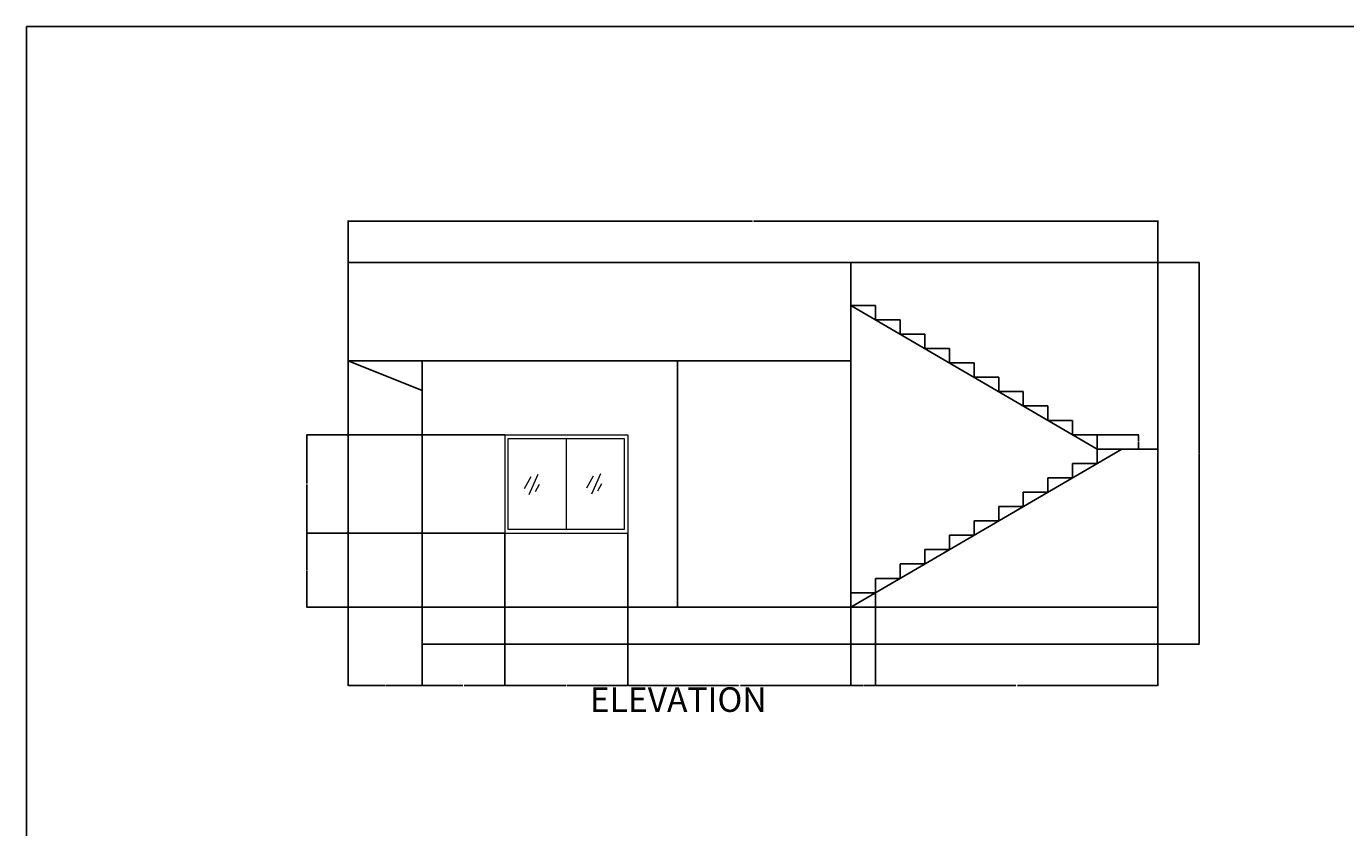
# Model space of a CAD drawing. Units: inches. Extents: x 1587 to 2880, y 1287 to 2423.
# Tile 5 of 8: x 1587 to 2229, y 2033 to 2423. Entities that reach past the tile are written whole.
import ezdxf

# ---------------------------------------------------------------- set-up
doc = ezdxf.new("R2010")
doc.units = ezdxf.units.IN
for name, color, linetype, lineweight in [('A-ANNO-DIMS', 2, 'Continuous', 18), ('A-ANNO-TEXT', 7, 'Continuous', 18), ('A-ANNO-TTLB', 7, 'Continuous', 25), ('A-ELEV', 7, 'Continuous', 25), ('A-FLOR-STRS', 7, 'Continuous', 25), ('A-GLAZ', 4, 'Continuous', 18)]:
    doc.layers.add(name, color=color, linetype=linetype, lineweight=lineweight)
doc.layers.add('A-WALL-PATT', color=251, linetype='Continuous', lineweight=13, true_color=0x636466)
doc.styles.get("Standard").update_dxf_attribs({"font": 'arial.ttf'})
doc.dimstyles.get("Standard").update_dxf_attribs({"dimtxt": 0.18, "dimasz": 0.18, "dimexe": 0.18, "dimexo": 0.0625, "dimgap": 0.09, "dimtad": 0, "dimtih": 1, "dimtoh": 1, "dimdec": 4, "dimzin": 0, "dimdsep": 46, "dimtxsty": 'Standard', "dimcen": 0.09, "dimadec": 0, "dimazin": 0, "dimtfac": 1, "dimtdec": 4, "dimtofl": 0, "dimtmove": 0, "dimatfit": 3, "dimfxl": 1, "dimtolj": 1, "dimtzin": 0, "dimarcsym": 0})

# ---------------------------------------------------------------- blocks, each defined once
blk = doc.blocks.new('GLASS-REFLECTION-ELEV')
for p, q in [((3.25, 8.8), (0, 2.81)), ((6.7, 9.88), (2.36, 0)), ((7.34, 5.04), (5.36, 1.47))]:
    blk.add_line(p, q)
blk = doc.blocks.new('*D82')
at = {"layer": 'A-ANNO-DIMS', "color": 0, "lineweight": -2, "transparency": 16777216}
for p, q in [((1743.34, 2308.21), (1743.34, 2328.48)), ((1743.52, 2328.3), (1940.2, 2328.3)), ((2137.66, 2328.3), (1940.99, 2328.3)), ((2137.84, 2308.21), (2137.84, 2328.48))]:
    blk.add_line(p, q, dxfattribs=at)
at = {"layer": 'A-ANNO-DIMS', "color": 0, "transparency": 16777216}
for points in [[(1743.52, 2328.33), (1743.52, 2328.27), (1743.34, 2328.3)], [(2137.66, 2328.33), (2137.66, 2328.27), (2137.84, 2328.3)]]:
    blk.add_solid(points, dxfattribs=at)
at = {"layer": 'Defpoints', "color": 0, "transparency": 16777216}
for p in [(2137.84, 2328.3), (1743.34, 2308.15), (2137.84, 2308.15)]:
    blk.add_point(p, dxfattribs=at)
at = {"layer": 'A-ANNO-DIMS', "color": 0, "transparency": 16777216, "insert": (1940.59, 2328.3), "char_height": 0.18, "attachment_point": 5}
blk.add_mtext('\\A1;394.5', dxfattribs=at)
blk = doc.blocks.new('*D83')
at = {"layer": 'A-ANNO-DIMS', "color": 0, "lineweight": -2, "transparency": 16777216}
for p, q in [((2137.9, 2308.15), (2158.17, 2308.15)), ((2157.99, 2307.97), (2157.99, 2215.33)), ((2157.99, 2122.33), (2157.99, 2214.97)), ((2137.9, 2122.15), (2158.17, 2122.15))]:
    blk.add_line(p, q, dxfattribs=at)
at = {"layer": 'A-ANNO-DIMS', "color": 0, "transparency": 16777216}
for points in [[(2157.96, 2307.97), (2158.02, 2307.97), (2157.99, 2308.15)], [(2157.96, 2122.33), (2158.02, 2122.33), (2157.99, 2122.15)]]:
    blk.add_solid(points, dxfattribs=at)
at = {"layer": 'Defpoints', "color": 0, "transparency": 16777216}
for p in [(2137.84, 2308.15), (2157.99, 2308.15), (2137.84, 2122.15)]:
    blk.add_point(p, dxfattribs=at)
at = {"layer": 'A-ANNO-DIMS', "color": 0, "transparency": 16777216, "insert": (2157.99, 2215.15), "char_height": 0.18, "attachment_point": 5}
blk.add_mtext('\\A1;186', dxfattribs=at)
blk = doc.blocks.new('*D84')
at = {"layer": 'A-ANNO-DIMS', "color": 0, "lineweight": -2, "transparency": 16777216}
for p, q in [((1743.34, 2260.09), (1743.34, 2101.82)), ((1779.34, 2122.09), (1779.34, 2101.82)), ((1743.52, 2102), (1761.12, 2102)), ((1779.16, 2102), (1761.56, 2102))]:
    blk.add_line(p, q, dxfattribs=at)
at = {"layer": 'A-ANNO-DIMS', "color": 0, "transparency": 16777216}
for points in [[(1743.52, 2102.03), (1743.52, 2101.97), (1743.34, 2102)], [(1779.16, 2102.03), (1779.16, 2101.97), (1779.34, 2102)]]:
    blk.add_solid(points, dxfattribs=at)
at = {"layer": 'Defpoints', "color": 0, "transparency": 16777216}
for p in [(1743.34, 2260.15), (1779.34, 2122.15), (1779.34, 2102)]:
    blk.add_point(p, dxfattribs=at)
at = {"layer": 'A-ANNO-DIMS', "color": 0, "transparency": 16777216, "insert": (1761.34, 2102), "char_height": 0.18, "attachment_point": 5}
blk.add_mtext('\\A1;36', dxfattribs=at)
blk = doc.blocks.new('*D85')
at = {"layer": 'A-ANNO-DIMS', "color": 0, "lineweight": -2, "transparency": 16777216}
for p, q in [((1819.66, 2176.09), (1819.66, 2101.82)), ((1779.34, 2140.09), (1779.34, 2101.82)), ((1779.52, 2102), (1799.11, 2102)), ((1819.48, 2102), (1799.9, 2102))]:
    blk.add_line(p, q, dxfattribs=at)
at = {"layer": 'A-ANNO-DIMS', "color": 0, "transparency": 16777216}
for points in [[(1779.52, 2102.03), (1779.52, 2101.97), (1779.34, 2102)], [(1819.48, 2102.03), (1819.48, 2101.97), (1819.66, 2102)]]:
    blk.add_solid(points, dxfattribs=at)
at = {"layer": 'Defpoints', "color": 0, "transparency": 16777216}
for p in [(1819.66, 2176.15), (1779.34, 2140.15), (1819.66, 2102)]:
    blk.add_point(p, dxfattribs=at)
at = {"layer": 'A-ANNO-DIMS', "color": 0, "transparency": 16777216, "insert": (1799.5, 2102), "char_height": 0.18, "attachment_point": 5}
blk.add_mtext('\\A1;40.32', dxfattribs=at)
blk = doc.blocks.new('*D86')
at = {"layer": 'A-ANNO-DIMS', "color": 0, "lineweight": -2, "transparency": 16777216}
for p, q in [((1819.66, 2176.09), (1819.66, 2101.82)), ((1879.66, 2176.09), (1879.66, 2101.82)), ((1819.84, 2102), (1849.44, 2102)), ((1879.48, 2102), (1849.88, 2102))]:
    blk.add_line(p, q, dxfattribs=at)
at = {"layer": 'A-ANNO-DIMS', "color": 0, "transparency": 16777216}
for points in [[(1819.84, 2102.03), (1819.84, 2101.97), (1819.66, 2102)], [(1879.48, 2102.03), (1879.48, 2101.97), (1879.66, 2102)]]:
    blk.add_solid(points, dxfattribs=at)
at = {"layer": 'Defpoints', "color": 0, "transparency": 16777216}
for p in [(1819.66, 2176.15), (1879.66, 2176.15), (1879.66, 2102)]:
    blk.add_point(p, dxfattribs=at)
at = {"layer": 'A-ANNO-DIMS', "color": 0, "transparency": 16777216, "insert": (1849.66, 2102), "char_height": 0.18, "attachment_point": 5}
blk.add_mtext('\\A1;60', dxfattribs=at)
blk = doc.blocks.new('*D87')
at = {"layer": 'A-ANNO-DIMS', "color": 0, "lineweight": -2, "transparency": 16777216}
for p, q in [((1879.66, 2176.09), (1879.66, 2101.82)), ((1988.29, 2140.09), (1988.29, 2101.82)), ((1879.84, 2102), (1933.52, 2102)), ((1988.11, 2102), (1934.43, 2102))]:
    blk.add_line(p, q, dxfattribs=at)
at = {"layer": 'A-ANNO-DIMS', "color": 0, "transparency": 16777216}
for points in [[(1879.84, 2102.03), (1879.84, 2101.97), (1879.66, 2102)], [(1988.11, 2102.03), (1988.11, 2101.97), (1988.29, 2102)]]:
    blk.add_solid(points, dxfattribs=at)
at = {"layer": 'Defpoints', "color": 0, "transparency": 16777216}
for p in [(1879.66, 2176.15), (1988.29, 2140.15), (1988.29, 2102)]:
    blk.add_point(p, dxfattribs=at)
at = {"layer": 'A-ANNO-DIMS', "color": 0, "transparency": 16777216, "insert": (1933.98, 2102), "char_height": 0.18, "attachment_point": 5}
blk.add_mtext('\\A1;108.63', dxfattribs=at)
blk = doc.blocks.new('*D88')
at = {"layer": 'A-ANNO-DIMS', "color": 0, "lineweight": -2, "transparency": 16777216}
for p, q in [((1819.6, 2224.15), (1723.01, 2224.15)), ((1723.19, 2223.97), (1723.19, 2200.33)), ((1723.19, 2176.33), (1723.19, 2199.97)), ((1819.6, 2176.15), (1723.01, 2176.15))]:
    blk.add_line(p, q, dxfattribs=at)
at = {"layer": 'A-ANNO-DIMS', "color": 0, "transparency": 16777216}
for points in [[(1723.16, 2223.97), (1723.22, 2223.97), (1723.19, 2224.15)], [(1723.16, 2176.33), (1723.22, 2176.33), (1723.19, 2176.15)]]:
    blk.add_solid(points, dxfattribs=at)
at = {"layer": 'Defpoints', "color": 0, "transparency": 16777216}
for p in [(1723.19, 2224.15), (1819.66, 2224.15), (1819.66, 2176.15)]:
    blk.add_point(p, dxfattribs=at)
at = {"layer": 'A-ANNO-DIMS', "color": 0, "transparency": 16777216, "insert": (1723.19, 2200.15), "char_height": 0.18, "attachment_point": 5}
blk.add_mtext('\\A1;48', dxfattribs=at)
blk = doc.blocks.new('*D89')
at = {"layer": 'A-ANNO-DIMS', "color": 0, "lineweight": -2, "transparency": 16777216}
for p, q in [((1819.6, 2176.15), (1723.01, 2176.15)), ((1723.19, 2175.97), (1723.19, 2158.33)), ((1723.19, 2140.33), (1723.19, 2157.97)), ((1779.28, 2140.15), (1723.01, 2140.15))]:
    blk.add_line(p, q, dxfattribs=at)
at = {"layer": 'A-ANNO-DIMS', "color": 0, "transparency": 16777216}
for points in [[(1723.16, 2175.97), (1723.22, 2175.97), (1723.19, 2176.15)], [(1723.16, 2140.33), (1723.22, 2140.33), (1723.19, 2140.15)]]:
    blk.add_solid(points, dxfattribs=at)
at = {"layer": 'Defpoints', "color": 0, "transparency": 16777216}
for p in [(1723.19, 2176.15), (1819.66, 2176.15), (1779.34, 2140.15)]:
    blk.add_point(p, dxfattribs=at)
at = {"layer": 'A-ANNO-DIMS', "color": 0, "transparency": 16777216, "insert": (1723.19, 2158.15), "char_height": 0.18, "attachment_point": 5}
blk.add_mtext('\\A1;36', dxfattribs=at)
blk = doc.blocks.new('*D90')
at = {"layer": 'A-ANNO-DIMS', "color": 0, "lineweight": -2, "transparency": 16777216}
for p, q in [((1988.29, 2147.09), (1988.29, 2101.82)), ((2000.29, 2147.09), (2000.29, 2101.82)), ((1988.47, 2102), (1994.08, 2102)), ((2000.11, 2102), (1994.5, 2102))]:
    blk.add_line(p, q, dxfattribs=at)
at = {"layer": 'A-ANNO-DIMS', "color": 0, "transparency": 16777216}
for points in [[(1988.47, 2102.03), (1988.47, 2101.97), (1988.29, 2102)], [(2000.11, 2102.03), (2000.11, 2101.97), (2000.29, 2102)]]:
    blk.add_solid(points, dxfattribs=at)
at = {"layer": 'Defpoints', "color": 0, "transparency": 16777216}
for p in [(1988.29, 2147.15), (2000.29, 2147.15), (2000.29, 2102)]:
    blk.add_point(p, dxfattribs=at)
at = {"layer": 'A-ANNO-DIMS', "color": 0, "transparency": 16777216, "insert": (1994.29, 2102), "char_height": 0.18, "attachment_point": 5}
blk.add_mtext('\\A1;12', dxfattribs=at)
blk = doc.blocks.new('*D91')
at = {"layer": 'A-ANNO-DIMS', "color": 0, "lineweight": -2, "transparency": 16777216}
for p, q in [((2000.29, 2147.09), (2000.29, 2101.82)), ((2137.84, 2140.09), (2137.84, 2101.82)), ((2000.47, 2102), (2068.61, 2102)), ((2137.66, 2102), (2069.52, 2102))]:
    blk.add_line(p, q, dxfattribs=at)
at = {"layer": 'A-ANNO-DIMS', "color": 0, "transparency": 16777216}
for points in [[(2000.47, 2102.03), (2000.47, 2101.97), (2000.29, 2102)], [(2137.66, 2102.03), (2137.66, 2101.97), (2137.84, 2102)]]:
    blk.add_solid(points, dxfattribs=at)
at = {"layer": 'Defpoints', "color": 0, "transparency": 16777216}
for p in [(2000.29, 2147.15), (2137.84, 2140.15), (2137.84, 2102)]:
    blk.add_point(p, dxfattribs=at)
at = {"layer": 'A-ANNO-DIMS', "color": 0, "transparency": 16777216, "insert": (2069.07, 2102), "char_height": 0.18, "attachment_point": 5}
blk.add_mtext('\\A1;137.55', dxfattribs=at)
blk = doc.blocks.new('*D92')
at = {"layer": 'A-ANNO-DIMS', "color": 0, "lineweight": -2, "transparency": 16777216}
for p, q in [((2108.356572, 2224.151475), (2128.624072, 2224.151475)), ((2128.444072, 2223.971475), (2128.444072, 2220.831475)), ((2128.444072, 2217.331475), (2128.444072, 2220.471475)), ((2108.356572, 2217.151475), (2128.624072, 2217.151475))]:
    blk.add_line(p, q, dxfattribs=at)
at = {"layer": 'A-ANNO-DIMS', "color": 0, "transparency": 16777216}
for points in [[(2128.414072, 2223.971475), (2128.474072, 2223.971475), (2128.444072, 2224.151475)], [(2128.414072, 2217.331475), (2128.474072, 2217.331475), (2128.444072, 2217.151475)]]:
    blk.add_solid(points, dxfattribs=at)
at = {"layer": 'Defpoints', "color": 0, "transparency": 16777216}
for p in [(2108.294072, 2224.151475), (2108.294072, 2217.151475), (2128.444072, 2217.151475)]:
    blk.add_point(p, dxfattribs=at)
at = {"layer": 'A-ANNO-DIMS', "color": 0, "transparency": 16777216, "insert": (2128.444072, 2220.651475), "char_height": 0.18, "attachment_point": 5}
blk.add_mtext('\\A1;7', dxfattribs=at)

msp = doc.modelspace()

# ---------------------------------------------------------------- hatches: boundary and pattern name
at = {"layer": 'A-WALL-PATT'}
h = msp.add_hatch(color=256, dxfattribs=at)
h.dxf.hatch_style = 1
h.paths.add_polyline_path([(2190.3423, 1988.3868), (2181.3423, 1988.3868), (2137.8423, 1988.3868), (1779.3423, 1988.3868), (1779.3423, 1939.6287), (1788.3423, 1939.6287), (1788.3423, 1979.3868), (1956.3423, 1979.3868), (1956.3423, 1841.3868), (1948.4175, 1841.3868), (1948.4175, 1836.8868), (1968.256, 1836.8868), (1968.256, 1839.1368), (1968.256, 1841.3868), (1960.8423, 1841.3868), (1960.8423, 1979.3868), (2128.8423, 1979.3868), (2128.8423, 1971.4394), (2133.3423, 1971.4394), (2133.3423, 1979.3868), (2181.3423, 1979.3868), (2181.3423, 1895.3868), (2174.9842, 1895.3868), (2174.9842, 1886.3868), (2190.3423, 1886.3868), (2190.3423, 1895.3868)])
h.paths.add_polyline_path([(1788.3423, 1879.6287), (1779.3423, 1879.6287), (1779.3423, 1827.4437), (1788.3423, 1827.4437), (1788.3423, 1836.8868), (1839.8915, 1836.8868), (1839.8915, 1839.1368), (1839.8915, 1841.3868), (1788.3423, 1841.3868)])
h.paths.add_polyline_path([(1876.8423, 1836.8868), (1908.901, 1836.8868), (1908.901, 1839.1368), (1908.901, 1841.3868), (1866.9993, 1841.3868), (1866.9993, 1836.8868), (1872.3423, 1836.8868), (1872.3423, 1776.8868), (1788.3423, 1776.8868), (1788.3423, 1803.4437), (1779.3423, 1803.4437), (1779.3423, 1757.1447), (1788.3423, 1757.1447), (1788.3423, 1772.3868), (1872.3423, 1772.3868), (1872.3423, 1712.3868), (1867.9542, 1712.3868), (1867.9542, 1707.8868), (1876.8423, 1707.8868), (1876.8423, 1772.3868)])
h.paths.add_polyline_path([(1842.6206, 1710.1368), (1842.6206, 1712.3868), (1788.3423, 1712.3868), (1788.3423, 1733.1447), (1779.3423, 1733.1447), (1779.3423, 1678.6557), (1788.3423, 1678.6557), (1788.3423, 1707.8868), (1842.6206, 1707.8868)])
h.paths.add_polyline_path([(1912.8423, 1712.3868), (1908.3423, 1712.3868), (1876.8423, 1712.3868), (1876.8423, 1707.8868), (1908.3423, 1707.8868), (1908.3423, 1702.2679), (1912.8423, 1702.2679)])
h.paths.add_polyline_path([(2137.8423, 1844.5168), (2128.8423, 1844.5168), (2128.8423, 1841.3868), (2006.9533, 1841.3868), (2006.9533, 1836.8868), (2128.8423, 1836.8868), (2128.8423, 1832.632), (2137.8423, 1832.632)])
h.paths.add_polyline_path([(1997.6598, 1534.8868), (1997.6598, 1539.3868), (1912.8423, 1539.3868), (1912.8423, 1543.4794), (1903.8423, 1543.4794), (1903.8423, 1530.3868), (1997.6598, 1530.3868)])
h.paths.add_polyline_path([(1912.8423, 1666.7101), (1910.5923, 1666.7101), (1908.3423, 1666.7101), (1908.3423, 1587.8868), (1903.8423, 1587.8868), (1879.6624, 1587.8868), (1879.6624, 1578.8868), (1903.8423, 1578.8868), (1903.8423, 1574.5584), (1912.8423, 1574.5584), (1912.8423, 1578.8868), (1912.8423, 1587.8868)])
h.paths.add_polyline_path([(1788.3423, 1618.6557), (1779.3423, 1618.6557), (1779.3423, 1578.8868), (1819.6624, 1578.8868), (1819.6624, 1583.3868), (1819.6624, 1587.8868), (1788.3423, 1587.8868)])
h.paths.add_polyline_path([(2133.3423, 1945.4046), (2131.0923, 1945.4046), (2128.8423, 1945.4046), (2128.8423, 1880.5168), (2137.8423, 1880.5168), (2137.8423, 1886.3868), (2150.9842, 1886.3868), (2150.9842, 1890.8868), (2150.9842, 1895.3868), (2133.3423, 1895.3868)], flags=17)
h.paths.add_polyline_path([(2137.8423, 1788.9874), (2133.3423, 1788.9874), (2128.8423, 1788.9874), (2128.8423, 1699.8868), (2006.9533, 1699.8868), (2006.9533, 1695.3868), (2128.8423, 1695.3868), (2128.8423, 1539.3868), (2057.6598, 1539.3868), (2057.6598, 1530.3868), (2128.8423, 1530.3868), (2128.8423, 1461.3868), (1988.2941, 1461.3868), (1988.2941, 1452.3868), (2137.8423, 1452.3868), (2137.8423, 1530.3868)])
h.paths.add_polyline_path([(1866.9166, 1348.94), (2042.3313, 1348.94), (2042.3313, 1371.6078), (1866.9166, 1371.6078)], flags=9)
h.paths.add_polyline_path([(2758.0473, 2126.4845), (2848.522, 2126.4845), (2848.522, 2138.8487), (2758.0473, 2138.8487)], flags=9)
h.paths.add_polyline_path([(2742.9428, 2216.0014), (2782.483, 2216.0014), (2782.483, 2228.3657), (2742.9428, 2228.3657)], flags=9)
h.paths.add_polyline_path([(2749.234, 2261.9992), (2784.0963, 2261.9992), (2784.0963, 2274.3634), (2749.234, 2274.3634)], flags=9)
h.paths.add_polyline_path([(2733.8012, 2281.8262), (2817.7726, 2281.8262), (2817.7726, 2294.1904), (2733.8012, 2294.1904)], flags=9)
h.paths.add_polyline_path([(2422.857, 2073.081), (2531.34, 2073.081), (2531.34, 2097.8095), (2422.857, 2097.8095)], flags=9)
h.paths.add_polyline_path([(1856.7732, 2082.3109), (1956.866, 2082.3109), (1956.866, 2107.0394), (1856.7732, 2107.0394)], flags=9)
h.paths.add_polyline_path([(2777.4581, 1646.9437), (2794.6887, 1646.9437), (2794.6887, 1671.6723), (2777.4581, 1671.6723)], flags=9)
h.paths.add_polyline_path([(2585.5416, 1728.5169), (2655.2006, 1728.5169), (2655.2006, 1760.9057), (2585.5416, 1760.9057)], flags=9)
h.paths.add_polyline_path([(2554.1301, 1617.6432), (2608.2079, 1617.6432), (2608.2079, 1640.032), (2554.1301, 1640.032)], flags=9)
h.paths.add_polyline_path([(2359.8658, 1678.1191), (2437.8454, 1678.1191), (2437.8454, 1700.5079), (2359.8658, 1700.5079)], flags=9)
h.paths.add_polyline_path([(2392.0171, 1749.26), (2422.3411, 1749.26), (2422.3411, 1767.9173), (2392.0171, 1767.9173)], flags=9)
h.paths.add_polyline_path([(2391.9937, 1787.5799), (2422.3177, 1787.5799), (2422.3177, 1806.2373), (2391.9937, 1806.2373)], flags=9)
h.paths.add_polyline_path([(2707.7632, 1927.6903), (2738.1623, 1927.6903), (2738.1623, 1946.3477), (2707.7632, 1946.3477)], flags=9)
h.paths.add_polyline_path([(2581.5534, 1846.9887), (2635.6148, 1846.9887), (2635.6148, 1869.3775), (2581.5534, 1869.3775)], flags=9)
h.paths.add_polyline_path([(2382.3802, 1864.4978), (2436.4416, 1864.4978), (2436.4416, 1886.8866), (2382.3802, 1886.8866)], flags=9)
h.paths.add_polyline_path([(2023.35, 1728.5169), (2093.0089, 1728.5169), (2093.0089, 1760.9057), (2023.35, 1760.9057)], flags=25)
h.paths.add_polyline_path([(1991.9385, 1617.6432), (2046.0162, 1617.6432), (2046.0162, 1640.032), (1991.9385, 1640.032)], flags=25)
h.paths.add_polyline_path([(1791.1103, 1678.1191), (1869.0899, 1678.1191), (1869.0899, 1700.5079), (1791.1103, 1700.5079)], flags=9)
h.paths.add_polyline_path([(1829.8255, 1749.26), (1860.1495, 1749.26), (1860.1495, 1767.9173), (1829.8255, 1767.9173)], flags=25)
h.paths.add_polyline_path([(1829.8021, 1787.5799), (1860.1261, 1787.5799), (1860.1261, 1806.2373), (1829.8021, 1806.2373)], flags=25)
h.paths.add_polyline_path([(2145.5716, 1927.6903), (2175.9706, 1927.6903), (2175.9706, 1946.3477), (2145.5716, 1946.3477)], flags=25)
h.paths.add_polyline_path([(2019.3617, 1846.9887), (2073.4231, 1846.9887), (2073.4231, 1869.3775), (2019.3617, 1869.3775)], flags=25)
h.paths.add_polyline_path([(1820.1886, 1864.4978), (1874.25, 1864.4978), (1874.25, 1886.8866), (1820.1886, 1886.8866)], flags=25)

# ---------------------------------------------------------------- linework, layer by layer
at = {"layer": 'A-ANNO-TTLB'}
msp.add_lwpolyline([(1586.5185, 2423.1539), (2880.2062, 2423.1539), (2880.2062, 1286.9347), (1586.5185, 1286.9347)], close=True, dxfattribs=at)
at = {"layer": 'A-ELEV'}
for p, q in [((1743.3423, 2308.1515), (2137.8423, 2308.1515)), ((1743.3423, 2260.1515), (1743.3423, 2308.1515)), ((1988.2941, 2260.1515), (1988.2941, 2308.1515)), ((2137.8423, 2308.1515), (2137.8423, 2122.1515)), ((1743.3423, 2260.1515), (1988.2941, 2260.1515)), ((1743.3423, 2260.1515), (1779.3423, 2245.7309)), ((1779.3423, 2260.1515), (1779.3423, 2122.1515)), ((1903.8423, 2260.1515), (1903.8423, 2140.1515)), ((1988.2941, 2260.1515), (1988.2941, 2140.1515)), ((1779.3423, 2140.1515), (2137.8423, 2140.1515)), ((1779.3423, 2122.1515), (2137.8423, 2122.1515))]:
    msp.add_line(p, q, dxfattribs=at)
at = {"layer": 'A-FLOR-STRS'}
for p, q in [((2000.2941, 2287.1515), (1988.2941, 2287.1515)), ((2108.2941, 2217.1515), (1988.2941, 2287.1515)), ((2000.2941, 2280.1515), (2000.2941, 2287.1515)), ((2012.2941, 2280.1515), (2000.2941, 2280.1515)), ((2012.2941, 2273.1515), (2012.2941, 2280.1515)), ((2024.2941, 2273.1515), (2012.2941, 2273.1515)), ((2024.2941, 2266.1515), (2024.2941, 2273.1515)), ((2036.2941, 2266.1515), (2024.2941, 2266.1515)), ((2036.2941, 2259.1515), (2036.2941, 2266.1515)), ((2048.2941, 2259.1515), (2036.2941, 2259.1515)), ((2048.2941, 2252.1515), (2048.2941, 2259.1515)), ((2060.2941, 2252.1515), (2048.2941, 2252.1515)), ((2060.2941, 2245.1515), (2060.2941, 2252.1515)), ((2072.2941, 2245.1515), (2060.2941, 2245.1515)), ((2072.2941, 2238.1515), (2072.2941, 2245.1515)), ((2084.2941, 2238.1515), (2072.2941, 2238.1515)), ((2084.2941, 2231.1515), (2084.2941, 2238.1515)), ((2096.2941, 2231.1515), (2084.2941, 2231.1515)), ((2096.2941, 2224.1515), (2096.2941, 2231.1515)), ((2108.2941, 2224.1515), (2096.2941, 2224.1515)), ((2108.2941, 2217.1515), (2108.2941, 2224.1515)), ((2120.2941, 2217.1515), (1988.2941, 2140.1515)), ((2108.2941, 2210.1515), (2108.2941, 2217.1515)), ((2108.2941, 2217.1515), (2137.8423, 2217.1515)), ((2108.2941, 2217.1515), (2120.2941, 2217.1515)), ((2120.2941, 2217.1515), (2120.2941, 2217.1515)), ((2120.2941, 2217.1515), (2120.2941, 2217.1515)), ((2096.2941, 2203.1515), (2096.2941, 2210.1515)), ((2096.2941, 2210.1515), (2108.2941, 2210.1515)), ((2084.2941, 2196.1515), (2084.2941, 2203.1515)), ((2084.2941, 2203.1515), (2096.2941, 2203.1515)), ((2072.2941, 2189.1515), (2072.2941, 2196.1515)), ((2072.2941, 2196.1515), (2084.2941, 2196.1515)), ((2060.2941, 2182.1515), (2060.2941, 2189.1515)), ((2060.2941, 2189.1515), (2072.2941, 2189.1515)), ((2048.2941, 2175.1515), (2048.2941, 2182.1515)), ((2048.2941, 2182.1515), (2060.2941, 2182.1515)), ((2036.2941, 2168.1515), (2036.2941, 2175.1515)), ((2036.2941, 2175.1515), (2048.2941, 2175.1515)), ((2024.2941, 2161.1515), (2024.2941, 2168.1515)), ((2024.2941, 2168.1515), (2036.2941, 2168.1515)), ((2012.2941, 2154.1515), (2012.2941, 2161.1515)), ((2012.2941, 2161.1515), (2024.2941, 2161.1515)), ((2000.2941, 2147.1515), (2000.2941, 2154.1515)), ((2000.2941, 2154.1515), (2012.2941, 2154.1515)), ((1988.2941, 2140.1515), (1988.2941, 2147.1515)), ((1988.2941, 2147.1515), (2000.2941, 2147.1515))]:
    msp.add_line(p, q, dxfattribs=at)
at = {"layer": 'A-GLAZ'}
for p, q in [((1819.6624, 2224.1515), (1819.6624, 2176.1515)), ((1819.6624, 2224.1515), (1879.6624, 2224.1515)), ((1849.557, 2222.2754), (1849.557, 2177.929)), ((1879.6624, 2224.1515), (1879.6624, 2176.1515)), ((1819.6624, 2176.1515), (1879.6624, 2176.1515))]:
    msp.add_line(p, q, dxfattribs=at)
msp.add_lwpolyline([(1821.2818, 2222.2754), (1877.8323, 2222.2754), (1877.8323, 2177.929), (1821.2818, 2177.929)], close=True, dxfattribs=at)

# ---------------------------------------------------------------- block references
for p in [(1859.4919, 2195.217), (1829.0309, 2194.8982)]:
    msp.add_blockref('GLASS-REFLECTION-ELEV', p, dxfattribs=at)

# ---------------------------------------------------------------- texts
at = {"layer": 'A-ANNO-TEXT', "insert": (1861.0992, 2101.0763), "char_height": 12, "attachment_point": 1}
msp.add_mtext_dynamic_manual_height_columns('ELEVATION', width=193.434468, gutter_width=12.5, heights=[0], dxfattribs=at)

# ---------------------------------------------------------------- dimensions: what is measured, and where the dimension line sits
at = {"layer": 'A-ANNO-DIMS'}
for base, p1, p2, override, picture, middle in [((2137.8423, 2328.3015), (1743.3423, 2308.1515), (2137.8423, 2308.1515), {"dimdec": 1, "dimlfac": 1, "dimrnd": 0, "dimzin": 0, "dimdsep": 46, "dimlunit": 2}, '*D82', (1940.5923, 2328.3015)), ((1779.3423, 2102.0015), (1743.3423, 2260.1515), (1779.3423, 2122.1515), {"dimdec": 0, "dimlfac": 1, "dimrnd": 0, "dimzin": 0, "dimdsep": 46, "dimlunit": 2}, '*D84', (1761.3423, 2102.0015)), ((1819.6624, 2102.0015), (1779.3423, 2140.1515), (1819.6624, 2176.1515), {"dimdec": 2, "dimlfac": 1, "dimrnd": 0, "dimzin": 0, "dimdsep": 46, "dimlunit": 2}, '*D85', (1799.5023, 2102.0015)), ((1879.6624, 2102.0015), (1819.6624, 2176.1515), (1879.6624, 2176.1515), {"dimdec": 0, "dimlfac": 1, "dimrnd": 0, "dimzin": 0, "dimdsep": 46, "dimlunit": 2}, '*D86', (1849.6624, 2102.0015)), ((1988.2941, 2102.0015), (1879.6624, 2176.1515), (1988.2941, 2140.1515), {"dimdec": 2, "dimlfac": 1, "dimrnd": 0, "dimzin": 0, "dimdsep": 46, "dimlunit": 2}, '*D87', (1933.9782, 2102.0015)), ((2000.2941, 2102.0015), (1988.2941, 2147.1515), (2000.2941, 2147.1515), {"dimdec": 0, "dimlfac": 1, "dimrnd": 0, "dimzin": 0, "dimdsep": 46, "dimlunit": 2}, '*D90', (1994.2941, 2102.0015)), ((2137.8423, 2102.0015), (2000.2941, 2147.1515), (2137.8423, 2140.1515), {"dimdec": 2, "dimlfac": 1, "dimrnd": 0, "dimzin": 0, "dimdsep": 46, "dimlunit": 2}, '*D91', (2069.0682, 2102.0015))]:
    dim = msp.add_linear_dim(base=base, p1=p1, p2=p2, dimstyle='Standard', override=override, dxfattribs=at)
    dim.commit()
    dim.dimension.update_dxf_attribs({"geometry": picture, "text_midpoint": middle})
for base, p1, p2, angle, picture, middle in [((2157.9923, 2308.1515), (2137.8423, 2122.1515), (2137.8423, 2308.1515), 90, '*D83', (2157.9923, 2215.1515)), ((1723.1923, 2224.1515), (1819.6624, 2176.1515), (1819.6624, 2224.1515), 90, '*D88', (1723.1923, 2200.1515)), ((2128.4441, 2217.1515), (2108.2941, 2224.1515), (2108.2941, 2217.1515), 270, '*D92', (2128.4441, 2220.6515)), ((1723.1923, 2176.1515), (1779.3423, 2140.1515), (1819.6624, 2176.1515), 90, '*D89', (1723.1923, 2158.1515))]:
    dim = msp.add_linear_dim(base=base, p1=p1, p2=p2, angle=angle, dimstyle='Standard', override={"dimdec": 0, "dimlfac": 1, "dimrnd": 0, "dimzin": 0, "dimdsep": 46, "dimlunit": 2}, dxfattribs=at)
    dim.commit()
    dim.dimension.update_dxf_attribs({"geometry": picture, "text_midpoint": middle})

doc.saveas('drawing.dxf')
